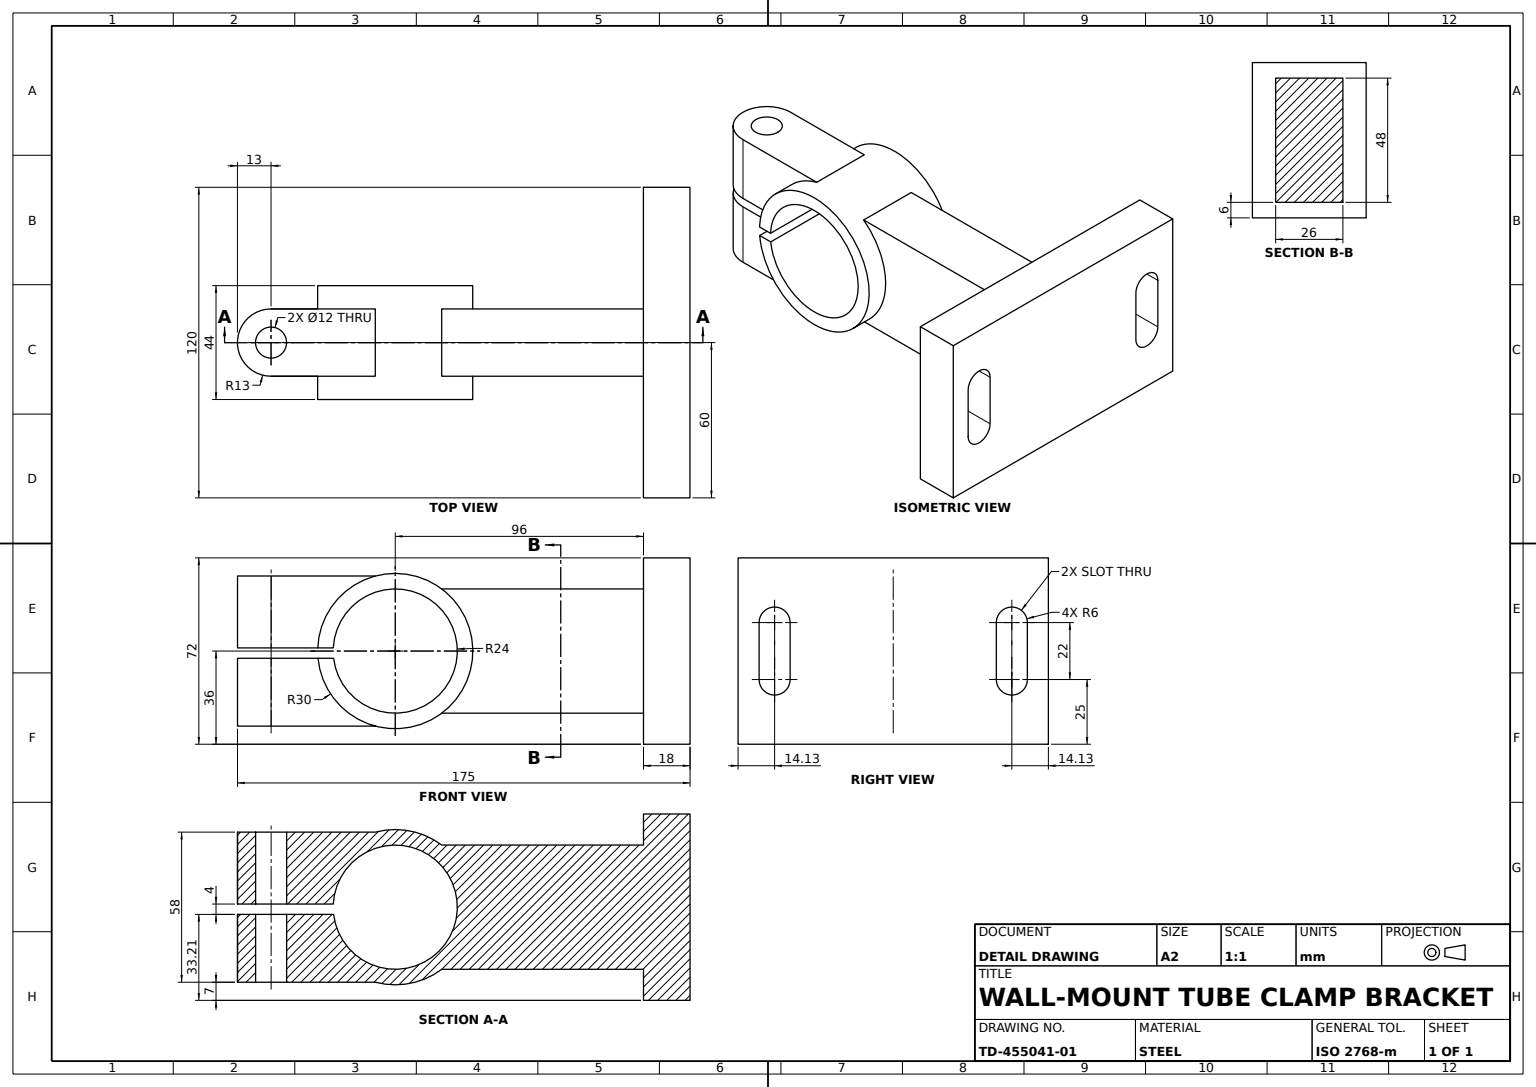
from build123d import *

# Parameters (mm, degrees)
BASE_PLATE_SKETCH_W        = 120
BASE_PLATE_SKETCH_H        = 72
BASE_PLATE_120X72X18_DEPTH = 9
CLAMP_RING_SKETCH_R        = 30
CLAMP_RING_SKETCH_R_2      = 24
CLAMP_RING_DEPTH           = 22
ARM_REACH                  = 190.308
ARM_END_RADIUS             = 30
ARM_PROFILE_SKETCH_W       = 26
ARM_PROFILE_SKETCH_H       = 48
CLAMP_LUG_DEPTH            = 13
CLAMP_LUG_EXTENSION_DEPTH  = 58
CLAMP_BOLT_HOLE_SKETCH_R   = 6
CLAMP_BOLT_HOLE_12_DEPTH   = 78
CLAMP_SPLIT_SLOT_SKETCH_W  = 44
CLAMP_SPLIT_SLOT_SKETCH_H  = 4
CLAMP_SPLIT_SLOT_4MM_DEPTH = 78
MOUNTING_SLOTS_2X_DEPTH    = 78


with BuildPart() as part:
    # Base Plate Sketch → Base Plate 120x72x18 (new, symmetric)
    with BuildSketch(Plane.XY):
        with Locations((60, 36)):
            Rectangle(BASE_PLATE_SKETCH_W, BASE_PLATE_SKETCH_H)
    extrude(amount=BASE_PLATE_120X72X18_DEPTH, both=True)



with BuildPart() as body_2:
    # Clamp Ring Sketch → Clamp Ring (new, symmetric)
    with BuildSketch(Plane(origin=(60, 0, 0), x_dir=(0, 0, -1), z_dir=(1, 0, 0))):
        with Locations(Location((-105, 36, 0), (0, 0, 180))):
            Circle(CLAMP_RING_SKETCH_R)
        with Locations(Location((-105, 36, 0), (0, 0, 180))):
            Circle(CLAMP_RING_SKETCH_R_2, mode=Mode.SUBTRACT)
    extrude(amount=CLAMP_RING_DEPTH, both=True)


with BuildPart() as part_1:
    add(part.part)

    add(body_2.part)  # Arm merges body 2
    # Arm: up to this cylinder (the profile starts outside it)
    arm_end = Plane(origin=(60, 36, 105), z_dir=(-1, 0, 0)) * Cylinder(ARM_END_RADIUS, 441.616, mode=Mode.PRIVATE)
    # Arm Profile Sketch → Arm (add, up to the surface)
    with BuildSketch(Plane.XY.offset(9), mode=Mode.PRIVATE) as arm_sk1:
        with Locations((60, 36)):
            Rectangle(ARM_PROFILE_SKETCH_W, ARM_PROFILE_SKETCH_H)
    arm_tool1 = extrude(arm_sk1.sketch, amount=ARM_REACH, mode=Mode.PRIVATE) - arm_end
    add(arm_tool1.solids().sort_by_distance((60, 36, 9))[0])

    # Clamp Lug Sketch → Clamp Lug (add, symmetric)
    with BuildSketch(Plane(origin=(60, 0, 0), x_dir=(0, 0, -1), z_dir=(1, 0, 0))):
        with BuildLine():
            Line((-153, 7), (-153, 65))
            Line((-153, 65), (-112.681145748, 65))
            ThreePointArc((-112.681145748, 65), (-135, 36), (-112.681145748, 7))
            Line((-112.681145748, 7), (-153, 7))
        make_face()
    extrude(amount=CLAMP_LUG_DEPTH, both=True)

    # Clamp Lug Extension Sketch → Clamp Lug Extension (add)
    with BuildSketch(Plane.XZ.offset(-7)):
        with BuildLine():
            Line((47, 153), (73, 153))
            ThreePointArc((73, 153), (60, 166), (47, 153))
        make_face()
    extrude(amount=-CLAMP_LUG_EXTENSION_DEPTH)

    # Clamp Bolt Hole Sketch → Clamp Bolt Hole Ø12 (cut)
    with BuildSketch(Plane.XZ.offset(-7)):
        with Locations(Location((60, 153, 0), (0, 0, 270))):
            Circle(CLAMP_BOLT_HOLE_SKETCH_R)
    extrude(amount=-CLAMP_BOLT_HOLE_12_DEPTH, mode=Mode.SUBTRACT)

    # Clamp Split Slot Sketch → Clamp Split Slot 4mm (cut)
    with BuildSketch(Plane.XY.offset(166)):
        with Locations((60, 35.211886187)):
            Rectangle(CLAMP_SPLIT_SLOT_SKETCH_W, CLAMP_SPLIT_SLOT_SKETCH_H)
    extrude(amount=-CLAMP_SPLIT_SLOT_4MM_DEPTH, mode=Mode.SUBTRACT)

    # Mounting Slots Sketch → Mounting Slots 2x (cut)
    with BuildSketch(Plane.XY.offset(9)):
        with BuildLine():
            Line((20.132428188, 47), (20.132428188, 25))
            ThreePointArc((20.132428188, 25), (14.132428188, 19), (8.132428188, 25))
            Line((8.132428188, 25), (8.132428188, 47))
            ThreePointArc((8.132428188, 47), (14.132428188, 53), (20.132428188, 47))
        make_face()
        with BuildLine():
            Line((99.867571812, 47), (99.867571812, 25))
            ThreePointArc((99.867571812, 25), (105.867571812, 19), (111.867571812, 25))
            Line((111.867571812, 25), (111.867571812, 47))
            ThreePointArc((111.867571812, 47), (105.867571812, 53), (99.867571812, 47))
        make_face()
    extrude(amount=-MOUNTING_SLOTS_2X_DEPTH, mode=Mode.SUBTRACT)


solid = part_1.part
